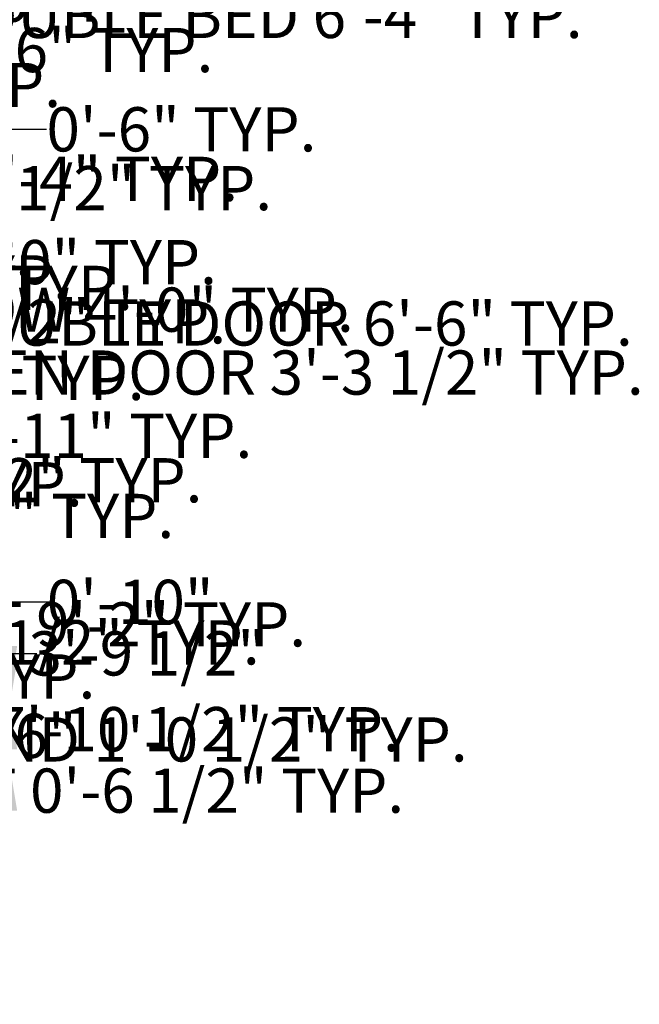
# Model space of a CAD drawing. Units: inches. Extents: x 7323 to 9737, y 2037 to 3322.
# Tile 16 of 19: x 9314 to 9737, y 2037 to 2709. Entities that reach past the tile are written whole.
import ezdxf

# ---------------------------------------------------------------- set-up
doc = ezdxf.new("R2010")
doc.units = ezdxf.units.IN
doc.header["$MEASUREMENT"] = 0
doc.layers.add('A-ANNO-DIMS', color=2, linetype='Continuous', lineweight=18)
doc.styles.get("Standard").update_dxf_attribs({"font": 'arial.ttf'})
doc.dimstyles.get("Standard").update_dxf_attribs({"dimtxt": 30.18, "dimasz": 30.18, "dimexe": 0.18, "dimexo": 0.0625, "dimgap": 0.09, "dimtad": 0, "dimtih": 1, "dimtoh": 1, "dimdec": 0, "dimzin": 0, "dimdsep": 46, "dimlunit": 3, "dimtxsty": 'Standard', "dimcen": 0.09, "dimadec": 0, "dimazin": 0, "dimtfac": 1, "dimtdec": 0, "dimtofl": 0, "dimtmove": 0, "dimatfit": 3, "dimfxl": 1, "dimtolj": 1, "dimtzin": 0, "dimarcsym": 0})

# ---------------------------------------------------------------- blocks, each defined once
blk = doc.blocks.new('*D35')
at = {"layer": 'A-ANNO-DIMS', "color": 0, "lineweight": -2, "transparency": 16777216}
for p, q in [((8977.7, 2688.2), (8947.52, 2688.2)), ((9007.88, 2687.36), (9007.88, 2688.38)), ((9013.95, 2687.36), (9013.95, 2688.38)), ((9044.13, 2688.2), (9074.31, 2688.2))]:
    blk.add_line(p, q, dxfattribs=at)
at = {"layer": 'A-ANNO-DIMS', "color": 0, "transparency": 16777216}
for points in [[(8977.7, 2693.23), (8977.7, 2683.17), (9007.88, 2688.2)], [(9044.13, 2693.23), (9044.13, 2683.17), (9013.95, 2688.2)]]:
    blk.add_solid(points, dxfattribs=at)
at = {"layer": 'Defpoints', "color": 0, "transparency": 16777216}
for p in [(9013.95, 2688.2), (9007.88, 2687.3), (9013.95, 2687.3)]:
    blk.add_point(p, dxfattribs=at)
at = {"layer": 'A-ANNO-DIMS', "color": 0, "transparency": 16777216, "insert": (9263.41, 2688.2), "char_height": 30.18, "attachment_point": 5}
blk.add_mtext('\\A1;COLUMN 0\'-6" TYP.', dxfattribs=at)
blk = doc.blocks.new('*D37')
at = {"layer": 'A-ANNO-DIMS', "color": 0, "lineweight": -2, "transparency": 16777216}
for p, q in [((9279.75, 2656.48), (9279.75, 2686.66)), ((9272.01, 2626.3), (9279.93, 2626.3)), ((9272.01, 2574.3), (9279.93, 2574.3)), ((9279.75, 2544.12), (9279.75, 2513.94))]:
    blk.add_line(p, q, dxfattribs=at)
at = {"layer": 'A-ANNO-DIMS', "color": 0, "transparency": 16777216}
for points in [[(9274.72, 2656.48), (9284.78, 2656.48), (9279.75, 2626.3)], [(9274.72, 2544.12), (9284.78, 2544.12), (9279.75, 2574.3)]]:
    blk.add_solid(points, dxfattribs=at)
at = {"layer": 'Defpoints', "color": 0, "transparency": 16777216}
for p in [(9271.95, 2626.3), (9271.95, 2574.3), (9279.75, 2574.3)]:
    blk.add_point(p, dxfattribs=at)
at = {"layer": 'A-ANNO-DIMS', "color": 0, "transparency": 16777216, "insert": (9279.75, 2600.3), "char_height": 30.18, "attachment_point": 5}
blk.add_mtext('\\A1;WINDOW 4\'-4" TYP.', dxfattribs=at)
blk = doc.blocks.new('*D38')
at = {"layer": 'A-ANNO-DIMS', "color": 0, "lineweight": -2, "transparency": 16777216}
for p, q in [((9235.77, 2634.1), (9205.59, 2634.1)), ((9265.95, 2626.36), (9265.95, 2634.28)), ((9271.95, 2626.36), (9271.95, 2634.28)), ((9302.13, 2634.1), (9332.31, 2634.1))]:
    blk.add_line(p, q, dxfattribs=at)
at = {"layer": 'A-ANNO-DIMS', "color": 0, "transparency": 16777216}
for points in [[(9235.77, 2639.13), (9235.77, 2629.07), (9265.95, 2634.1)], [(9302.13, 2639.13), (9302.13, 2629.07), (9271.95, 2634.1)]]:
    blk.add_solid(points, dxfattribs=at)
at = {"layer": 'Defpoints', "color": 0, "transparency": 16777216}
for p in [(9271.95, 2634.1), (9265.95, 2626.3), (9271.95, 2626.3)]:
    blk.add_point(p, dxfattribs=at)
at = {"layer": 'A-ANNO-DIMS', "color": 0, "transparency": 16777216, "insert": (9424.38, 2634.1), "char_height": 30.18, "attachment_point": 5}
blk.add_mtext('\\A1;0\'-6" TYP.', dxfattribs=at)
blk = doc.blocks.new('*D39')
at = {"layer": 'A-ANNO-DIMS', "color": 0, "lineweight": -2, "transparency": 16777216}
for p, q in [((8647.94, 2549.03), (8617.76, 2549.03)), ((8678.12, 2543.2), (8678.12, 2549.21)), ((8717.39, 2543.2), (8717.39, 2549.21)), ((8747.57, 2549.03), (8777.75, 2549.03))]:
    blk.add_line(p, q, dxfattribs=at)
at = {"layer": 'A-ANNO-DIMS', "color": 0, "transparency": 16777216}
for points in [[(8647.94, 2554.06), (8647.94, 2544), (8678.12, 2549.03)], [(8747.57, 2554.06), (8747.57, 2544), (8717.39, 2549.03)]]:
    blk.add_solid(points, dxfattribs=at)
at = {"layer": 'Defpoints', "color": 0, "transparency": 16777216}
for p in [(8717.39, 2549.03), (8678.12, 2543.14), (8717.39, 2543.14)]:
    blk.add_point(p, dxfattribs=at)
at = {"layer": 'A-ANNO-DIMS', "color": 0, "transparency": 16777216, "insert": (9057.19, 2549.03), "char_height": 30.18, "attachment_point": 5}
blk.add_mtext('\\A1;SINGLE DOOR 3\'-3 1/2" TYP.', dxfattribs=at)
blk = doc.blocks.new('*D43')
at = {"layer": 'A-ANNO-DIMS', "color": 0, "lineweight": -2, "transparency": 16777216}
for p, q in [((9108.94, 2438.75), (9108.94, 2468.93)), ((9104.01, 2408.57), (9109.12, 2408.57)), ((9104.01, 2375.3), (9109.12, 2375.3)), ((9108.94, 2345.12), (9108.94, 2314.94))]:
    blk.add_line(p, q, dxfattribs=at)
at = {"layer": 'A-ANNO-DIMS', "color": 0, "transparency": 16777216}
for points in [[(9103.91, 2438.75), (9113.97, 2438.75), (9108.94, 2408.57)], [(9103.91, 2345.12), (9113.97, 2345.12), (9108.94, 2375.3)]]:
    blk.add_solid(points, dxfattribs=at)
at = {"layer": 'Defpoints', "color": 0, "transparency": 16777216}
for p in [(9103.95, 2408.57), (9108.94, 2408.57), (9103.95, 2375.3)]:
    blk.add_point(p, dxfattribs=at)
at = {"layer": 'A-ANNO-DIMS', "color": 0, "transparency": 16777216, "insert": (9108.94, 2391.93), "char_height": 30.18, "attachment_point": 5}
blk.add_mtext('\\A1;BATH DOOR 2\'-9 1/2" TYP.', dxfattribs=at)
blk = doc.blocks.new('*D44')
at = {"layer": 'A-ANNO-DIMS', "color": 0, "lineweight": -2, "transparency": 16777216}
for p, q in [((9070.67, 2375.23), (9070.67, 2370.12)), ((9103.95, 2375.23), (9103.95, 2370.12)), ((9040.49, 2370.3), (9010.31, 2370.3)), ((9134.13, 2370.3), (9164.31, 2370.3))]:
    blk.add_line(p, q, dxfattribs=at)
at = {"layer": 'A-ANNO-DIMS', "color": 0, "transparency": 16777216}
for points in [[(9040.49, 2375.33), (9040.49, 2365.27), (9070.67, 2370.3)], [(9134.13, 2375.33), (9134.13, 2365.27), (9103.95, 2370.3)]]:
    blk.add_solid(points, dxfattribs=at)
at = {"layer": 'Defpoints', "color": 0, "transparency": 16777216}
for p in [(9070.67, 2375.3), (9103.95, 2375.3), (9103.95, 2370.3)]:
    blk.add_point(p, dxfattribs=at)
at = {"layer": 'A-ANNO-DIMS', "color": 0, "transparency": 16777216, "insert": (9291.8, 2370.3), "char_height": 30.18, "attachment_point": 5}
blk.add_mtext('\\A1;2\'-9 1/2" TYP.', dxfattribs=at)
blk = doc.blocks.new('*D45')
at = {"layer": 'A-ANNO-DIMS', "color": 0, "lineweight": -2, "transparency": 16777216}
for p, q in [((8725.79, 2664.36), (8695.61, 2664.36)), ((8755.97, 2662.02), (8755.97, 2664.54)), ((8772, 2662.02), (8772, 2664.54)), ((8802.18, 2664.36), (8832.36, 2664.36))]:
    blk.add_line(p, q, dxfattribs=at)
at = {"layer": 'A-ANNO-DIMS', "color": 0, "transparency": 16777216}
for points in [[(8725.79, 2669.39), (8725.79, 2659.33), (8755.97, 2664.36)], [(8802.18, 2669.39), (8802.18, 2659.33), (8772, 2664.36)]]:
    blk.add_solid(points, dxfattribs=at)
at = {"layer": 'Defpoints', "color": 0, "transparency": 16777216}
for p in [(8755.97, 2661.96), (8772, 2664.36), (8772, 2661.96)]:
    blk.add_point(p, dxfattribs=at)
at = {"layer": 'A-ANNO-DIMS', "color": 0, "transparency": 16777216, "insert": (9094.8, 2664.36), "char_height": 30.18, "attachment_point": 5}
blk.add_mtext('\\A1;BEDSIDE TABLE 1\'-4" TYP.', dxfattribs=at)
blk = doc.blocks.new('*D47')
at = {"layer": 'A-ANNO-DIMS', "color": 0, "lineweight": -2, "transparency": 16777216}
for p, q in [((8809.55, 2464.49), (8779.37, 2464.49)), ((8839.73, 2461.79), (8839.73, 2464.67)), ((8858.14, 2461.79), (8858.14, 2464.67)), ((8888.32, 2464.49), (8918.5, 2464.49))]:
    blk.add_line(p, q, dxfattribs=at)
at = {"layer": 'A-ANNO-DIMS', "color": 0, "transparency": 16777216}
for points in [[(8809.55, 2469.52), (8809.55, 2459.46), (8839.73, 2464.49)], [(8888.32, 2469.52), (8888.32, 2459.46), (8858.14, 2464.49)]]:
    blk.add_solid(points, dxfattribs=at)
at = {"layer": 'Defpoints', "color": 0, "transparency": 16777216}
for p in [(8839.73, 2461.73), (8858.14, 2464.49), (8858.14, 2461.73)]:
    blk.add_point(p, dxfattribs=at)
at = {"layer": 'A-ANNO-DIMS', "color": 0, "transparency": 16777216, "insert": (9164.9, 2464.49), "char_height": 30.18, "attachment_point": 5}
blk.add_mtext('\\A1;ARMCHAIR 1\'-6 1/2" TYP.', dxfattribs=at)
blk = doc.blocks.new('*D49')
at = {"layer": 'A-ANNO-DIMS', "color": 0, "lineweight": -2, "transparency": 16777216}
for p, q in [((8908.77, 2183.8), (8908.77, 2182.67)), ((8915.5, 2183.8), (8915.5, 2182.67)), ((8878.59, 2182.85), (8848.41, 2182.85)), ((8945.68, 2182.85), (8975.86, 2182.85))]:
    blk.add_line(p, q, dxfattribs=at)
at = {"layer": 'A-ANNO-DIMS', "color": 0, "transparency": 16777216}
for points in [[(8878.59, 2187.88), (8878.59, 2177.82), (8908.77, 2182.85)], [(8945.68, 2187.88), (8945.68, 2177.82), (8915.5, 2182.85)]]:
    blk.add_solid(points, dxfattribs=at)
at = {"layer": 'Defpoints', "color": 0, "transparency": 16777216}
for p in [(8908.77, 2183.86), (8915.5, 2183.86), (8915.5, 2182.85)]:
    blk.add_point(p, dxfattribs=at)
at = {"layer": 'A-ANNO-DIMS', "color": 0, "transparency": 16777216, "insert": (9284.58, 2182.85), "char_height": 30.18, "attachment_point": 5}
blk.add_mtext('\\A1;STAIR END POST 0\'-6 1/2" TYP.', dxfattribs=at)
blk = doc.blocks.new('*D51')
at = {"layer": 'A-ANNO-DIMS', "color": 0, "lineweight": -2, "transparency": 16777216}
for p, q in [((9130.95, 2513.23), (9130.95, 2501.42)), ((9208.95, 2513.23), (9208.95, 2501.42)), ((9161.13, 2501.6), (9178.77, 2501.6)), ((9208.95, 2501.6), (9239.13, 2501.6))]:
    blk.add_line(p, q, dxfattribs=at)
at = {"layer": 'A-ANNO-DIMS', "color": 0, "transparency": 16777216}
for points in [[(9161.13, 2506.63), (9161.13, 2496.57), (9130.95, 2501.6)], [(9178.77, 2506.63), (9178.77, 2496.57), (9208.95, 2501.6)]]:
    blk.add_solid(points, dxfattribs=at)
at = {"layer": 'Defpoints', "color": 0, "transparency": 16777216}
for p in [(9130.95, 2513.3), (9208.95, 2513.3), (9208.95, 2501.6)]:
    blk.add_point(p, dxfattribs=at)
at = {"layer": 'A-ANNO-DIMS', "color": 0, "transparency": 16777216, "insert": (9492.09, 2501.6), "char_height": 30.18, "attachment_point": 5}
blk.add_mtext('\\A1;DOUBLE DOOR 6\'-6" TYP.', dxfattribs=at)
blk = doc.blocks.new('*D52')
at = {"layer": 'A-ANNO-DIMS', "color": 0, "lineweight": -2, "transparency": 16777216}
for p, q in [((9220.65, 2583.03), (9220.65, 2613.21)), ((9209.01, 2552.85), (9220.83, 2552.85)), ((9209.01, 2513.3), (9220.83, 2513.3)), ((9220.65, 2483.12), (9220.65, 2452.94))]:
    blk.add_line(p, q, dxfattribs=at)
at = {"layer": 'A-ANNO-DIMS', "color": 0, "transparency": 16777216}
for points in [[(9215.62, 2583.03), (9225.68, 2583.03), (9220.65, 2552.85)], [(9215.62, 2483.12), (9225.68, 2483.12), (9220.65, 2513.3)]]:
    blk.add_solid(points, dxfattribs=at)
at = {"layer": 'Defpoints', "color": 0, "transparency": 16777216}
for p in [(9208.95, 2552.85), (9220.65, 2552.85), (9208.95, 2513.3)]:
    blk.add_point(p, dxfattribs=at)
at = {"layer": 'A-ANNO-DIMS', "color": 0, "transparency": 16777216, "insert": (9220.65, 2533.07), "char_height": 30.18, "attachment_point": 5}
blk.add_mtext('\\A1;3\'-3 1/2" TYP.', dxfattribs=at)
blk = doc.blocks.new('*D53')
at = {"layer": 'A-ANNO-DIMS', "color": 0, "lineweight": -2, "transparency": 16777216}
for p, q in [((8826.85, 2511.06), (8796.67, 2511.06)), ((8857.03, 2503.93), (8857.03, 2511.24)), ((8905.03, 2503.93), (8905.03, 2511.24)), ((8935.21, 2511.06), (8965.39, 2511.06))]:
    blk.add_line(p, q, dxfattribs=at)
at = {"layer": 'A-ANNO-DIMS', "color": 0, "transparency": 16777216}
for points in [[(8826.85, 2516.09), (8826.85, 2506.03), (8857.03, 2511.06)], [(8935.21, 2516.09), (8935.21, 2506.03), (8905.03, 2511.06)]]:
    blk.add_solid(points, dxfattribs=at)
at = {"layer": 'Defpoints', "color": 0, "transparency": 16777216}
for p in [(8905.03, 2511.06), (8857.03, 2503.86), (8905.03, 2503.86)]:
    blk.add_point(p, dxfattribs=at)
at = {"layer": 'A-ANNO-DIMS', "color": 0, "transparency": 16777216, "insert": (9261.3, 2511.06), "char_height": 30.18, "attachment_point": 5}
blk.add_mtext('\\A1;INTERIOR WINDOW 4\'-0" TYP.', dxfattribs=at)
blk = doc.blocks.new('*D55')
at = {"layer": 'A-ANNO-DIMS', "color": 0, "lineweight": -2, "transparency": 16777216}
for p, q in [((9265.38, 2351.3), (9282, 2351.3)), ((9281.82, 2321.12), (9281.82, 2311.99)), ((9281.82, 2271.48), (9281.82, 2280.6)), ((9265.38, 2241.3), (9282, 2241.3))]:
    blk.add_line(p, q, dxfattribs=at)
at = {"layer": 'A-ANNO-DIMS', "color": 0, "transparency": 16777216}
for points in [[(9276.79, 2321.12), (9286.85, 2321.12), (9281.82, 2351.3)], [(9276.79, 2271.48), (9286.85, 2271.48), (9281.82, 2241.3)]]:
    blk.add_solid(points, dxfattribs=at)
at = {"layer": 'Defpoints', "color": 0, "transparency": 16777216}
for p in [(9265.32, 2351.3), (9281.82, 2351.3), (9265.32, 2241.3)]:
    blk.add_point(p, dxfattribs=at)
at = {"layer": 'A-ANNO-DIMS', "color": 0, "transparency": 16777216, "insert": (9281.82, 2296.3), "char_height": 30.18, "attachment_point": 5}
blk.add_mtext('\\A1;STAIR FLIGHT 9\'-2" TYP.', dxfattribs=at)
blk = doc.blocks.new('*D56')
at = {"layer": 'A-ANNO-DIMS', "color": 0, "lineweight": -2, "transparency": 16777216}
for p, q in [((9170.68, 2241.23), (9170.68, 2224.62)), ((9265.32, 2241.23), (9265.32, 2224.62)), ((9200.86, 2224.8), (9235.14, 2224.8)), ((9265.32, 2224.8), (9295.5, 2224.8))]:
    blk.add_line(p, q, dxfattribs=at)
at = {"layer": 'A-ANNO-DIMS', "color": 0, "transparency": 16777216}
for points in [[(9200.86, 2229.83), (9200.86, 2219.77), (9170.68, 2224.8)], [(9235.14, 2229.83), (9235.14, 2219.77), (9265.32, 2224.8)]]:
    blk.add_solid(points, dxfattribs=at)
at = {"layer": 'Defpoints', "color": 0, "transparency": 16777216}
for p in [(9170.68, 2241.3), (9265.32, 2241.3), (9265.32, 2224.8)]:
    blk.add_point(p, dxfattribs=at)
at = {"layer": 'A-ANNO-DIMS', "color": 0, "transparency": 16777216, "insert": (9434.33, 2224.8), "char_height": 30.18, "attachment_point": 5}
blk.add_mtext('\\A1;7\'-10 1/2" TYP.', dxfattribs=at)
blk = doc.blocks.new('*D59')
at = {"layer": 'A-ANNO-DIMS', "color": 0, "lineweight": -2, "transparency": 16777216}
for p, q in [((9064.67, 2473.96), (9064.67, 2467.95)), ((9103.95, 2473.96), (9103.95, 2467.95)), ((9034.49, 2468.13), (9004.31, 2468.13)), ((9134.13, 2468.13), (9164.31, 2468.13))]:
    blk.add_line(p, q, dxfattribs=at)
at = {"layer": 'A-ANNO-DIMS', "color": 0, "transparency": 16777216}
for points in [[(9034.49, 2473.16), (9034.49, 2463.1), (9064.67, 2468.13)], [(9134.13, 2473.16), (9134.13, 2463.1), (9103.95, 2468.13)]]:
    blk.add_solid(points, dxfattribs=at)
at = {"layer": 'Defpoints', "color": 0, "transparency": 16777216}
for p in [(9064.67, 2474.02), (9103.95, 2474.02), (9103.95, 2468.13)]:
    blk.add_point(p, dxfattribs=at)
at = {"layer": 'A-ANNO-DIMS', "color": 0, "transparency": 16777216, "insert": (9458.35, 2468.13), "char_height": 30.18, "attachment_point": 5}
blk.add_mtext('\\A1;KITCHEN DOOR 3\'-3 1/2" TYP.', dxfattribs=at)
blk = doc.blocks.new('*D61')
at = {"layer": 'A-ANNO-DIMS', "color": 0, "lineweight": -2, "transparency": 16777216}
for p, q in [((9212.57, 2681.3), (9212.57, 2711.48)), ((9212.57, 2711.48), (9242.75, 2711.48)), ((9201.24, 2681.3), (9212.75, 2681.3)), ((9212.57, 2635.56), (9212.57, 2651.12)), ((9201.24, 2605.38), (9212.75, 2605.38))]:
    blk.add_line(p, q, dxfattribs=at)
at = {"layer": 'A-ANNO-DIMS', "color": 0, "transparency": 16777216}
for points in [[(9207.54, 2651.12), (9217.6, 2651.12), (9212.57, 2681.3)], [(9207.54, 2635.56), (9217.6, 2635.56), (9212.57, 2605.38)]]:
    blk.add_solid(points, dxfattribs=at)
at = {"layer": 'Defpoints', "color": 0, "transparency": 16777216}
for p in [(9201.18, 2681.3), (9212.57, 2681.3), (9201.18, 2605.38)]:
    blk.add_point(p, dxfattribs=at)
at = {"layer": 'A-ANNO-DIMS', "color": 0, "transparency": 16777216, "insert": (9475.82, 2711.48), "char_height": 30.18, "attachment_point": 5}
blk.add_mtext('\\A1;DOUBLE BED 6\'-4" TYP.', dxfattribs=at)
blk = doc.blocks.new('*D62')
at = {"layer": 'A-ANNO-DIMS', "color": 0, "lineweight": -2, "transparency": 16777216}
for p, q in [((9134.53, 2605.32), (9134.53, 2593.82)), ((9201.18, 2605.32), (9201.18, 2593.82)), ((9164.71, 2594), (9171, 2594)), ((9201.18, 2594), (9231.36, 2594))]:
    blk.add_line(p, q, dxfattribs=at)
at = {"layer": 'A-ANNO-DIMS', "color": 0, "transparency": 16777216}
for points in [[(9164.71, 2599.03), (9164.71, 2588.97), (9134.53, 2594)], [(9171, 2599.03), (9171, 2588.97), (9201.18, 2594)]]:
    blk.add_solid(points, dxfattribs=at)
at = {"layer": 'Defpoints', "color": 0, "transparency": 16777216}
for p in [(9134.53, 2605.38), (9201.18, 2605.38), (9201.18, 2594)]:
    blk.add_point(p, dxfattribs=at)
at = {"layer": 'A-ANNO-DIMS', "color": 0, "transparency": 16777216, "insert": (9358.59, 2594), "char_height": 30.18, "attachment_point": 5}
blk.add_mtext('\\A1;5\'-6 1/2" TYP.', dxfattribs=at)
blk = doc.blocks.new('*D65')
at = {"layer": 'A-ANNO-DIMS', "color": 0, "lineweight": -2, "transparency": 16777216}
for p, q in [((9024.02, 2513.3), (9024.02, 2543.48)), ((9024.02, 2543.48), (9054.2, 2543.48)), ((9036.56, 2513.3), (9023.84, 2513.3)), ((9024.02, 2459.48), (9024.02, 2483.12)), ((9036.56, 2429.3), (9023.84, 2429.3))]:
    blk.add_line(p, q, dxfattribs=at)
at = {"layer": 'A-ANNO-DIMS', "color": 0, "transparency": 16777216}
for points in [[(9018.99, 2483.12), (9029.05, 2483.12), (9024.02, 2513.3)], [(9018.99, 2459.48), (9029.05, 2459.48), (9024.02, 2429.3)]]:
    blk.add_solid(points, dxfattribs=at)
at = {"layer": 'Defpoints', "color": 0, "transparency": 16777216}
for p in [(9024.02, 2513.3), (9036.62, 2513.3), (9036.62, 2429.3)]:
    blk.add_point(p, dxfattribs=at)
at = {"layer": 'A-ANNO-DIMS', "color": 0, "transparency": 16777216, "insert": (9256.18, 2543.48), "char_height": 30.18, "attachment_point": 5}
blk.add_mtext('\\A1;COUNTER 7\'-0" TYP.', dxfattribs=at)
blk = doc.blocks.new('*D66')
at = {"layer": 'A-ANNO-DIMS', "color": 0, "lineweight": -2, "transparency": 16777216}
for p, q in [((9006.44, 2525.9), (8976.26, 2525.9)), ((9036.62, 2513.36), (9036.62, 2526.08)), ((9075.95, 2513.36), (9075.95, 2526.08)), ((9106.13, 2525.9), (9136.31, 2525.9))]:
    blk.add_line(p, q, dxfattribs=at)
at = {"layer": 'A-ANNO-DIMS', "color": 0, "transparency": 16777216}
for points in [[(9006.44, 2530.93), (9006.44, 2520.87), (9036.62, 2525.9)], [(9106.13, 2530.93), (9106.13, 2520.87), (9075.95, 2525.9)]]:
    blk.add_solid(points, dxfattribs=at)
at = {"layer": 'Defpoints', "color": 0, "transparency": 16777216}
for p in [(9075.95, 2525.9), (9036.62, 2513.3), (9075.95, 2513.3)]:
    blk.add_point(p, dxfattribs=at)
at = {"layer": 'A-ANNO-DIMS', "color": 0, "transparency": 16777216, "insert": (9263.53, 2525.9), "char_height": 30.18, "attachment_point": 5}
blk.add_mtext('\\A1;3\'-3 1/2" TYP.', dxfattribs=at)
blk = doc.blocks.new('*D67')
at = {"layer": 'A-ANNO-DIMS', "color": 0, "lineweight": -2, "transparency": 16777216}
for p, q in [((9145.07, 2308.82), (9145.07, 2339)), ((9150.37, 2278.64), (9144.89, 2278.64)), ((9150.37, 2242.89), (9144.89, 2242.89)), ((9145.07, 2212.71), (9145.07, 2182.53))]:
    blk.add_line(p, q, dxfattribs=at)
at = {"layer": 'A-ANNO-DIMS', "color": 0, "transparency": 16777216}
for points in [[(9140.04, 2308.82), (9150.1, 2308.82), (9145.07, 2278.64)], [(9140.04, 2212.71), (9150.1, 2212.71), (9145.07, 2242.89)]]:
    blk.add_solid(points, dxfattribs=at)
at = {"layer": 'Defpoints', "color": 0, "transparency": 16777216}
for p in [(9145.07, 2278.64), (9150.44, 2278.64), (9150.44, 2242.89)]:
    blk.add_point(p, dxfattribs=at)
at = {"layer": 'A-ANNO-DIMS', "color": 0, "transparency": 16777216, "insert": (9145.07, 2260.76), "char_height": 30.18, "attachment_point": 5}
blk.add_mtext('\\A1;TV UNIT 2\'-11 1/2" TYP.', dxfattribs=at)
blk = doc.blocks.new('*D68')
at = {"layer": 'A-ANNO-DIMS', "color": 0, "lineweight": -2, "transparency": 16777216}
for p, q in [((9120.26, 2284), (9090.08, 2284)), ((9150.44, 2278.7), (9150.44, 2284.18)), ((9163.95, 2278.7), (9163.95, 2284.18)), ((9194.13, 2284), (9224.31, 2284))]:
    blk.add_line(p, q, dxfattribs=at)
at = {"layer": 'A-ANNO-DIMS', "color": 0, "transparency": 16777216}
for points in [[(9120.26, 2289.03), (9120.26, 2278.97), (9150.44, 2284)], [(9194.13, 2289.03), (9194.13, 2278.97), (9163.95, 2284)]]:
    blk.add_solid(points, dxfattribs=at)
at = {"layer": 'Defpoints', "color": 0, "transparency": 16777216}
for p in [(9150.44, 2278.64), (9163.95, 2284), (9163.95, 2278.64)]:
    blk.add_point(p, dxfattribs=at)
at = {"layer": 'A-ANNO-DIMS', "color": 0, "transparency": 16777216, "insert": (9350.12, 2284), "char_height": 30.18, "attachment_point": 5}
blk.add_mtext('\\A1;1\'-1 1/2" TYP.', dxfattribs=at)
blk = doc.blocks.new('*D69')
at = {"layer": 'A-ANNO-DIMS', "color": 0, "lineweight": -2, "transparency": 16777216}
for p, q in [((8836.58, 2472.89), (8836.58, 2503.07)), ((8836.58, 2503.07), (8866.76, 2503.07)), ((8839.88, 2442.71), (8836.4, 2442.71)), ((8839.88, 2420.33), (8836.4, 2420.33)), ((8836.58, 2390.15), (8836.58, 2359.97))]:
    blk.add_line(p, q, dxfattribs=at)
at = {"layer": 'A-ANNO-DIMS', "color": 0, "transparency": 16777216}
for points in [[(8831.55, 2472.89), (8841.61, 2472.89), (8836.58, 2442.71)], [(8831.55, 2390.15), (8841.61, 2390.15), (8836.58, 2420.33)]]:
    blk.add_solid(points, dxfattribs=at)
at = {"layer": 'Defpoints', "color": 0, "transparency": 16777216}
for p in [(8836.58, 2442.71), (8839.94, 2442.71), (8839.94, 2420.33)]:
    blk.add_point(p, dxfattribs=at)
at = {"layer": 'A-ANNO-DIMS', "color": 0, "transparency": 16777216, "insert": (9169.54, 2503.07), "char_height": 30.18, "attachment_point": 5}
blk.add_mtext('\\A1;COFFEE TABLE 1\'-10 1/2" TYP.', dxfattribs=at)
blk = doc.blocks.new('*D73')
at = {"layer": 'A-ANNO-DIMS', "color": 0, "lineweight": -2, "transparency": 16777216}
for p, q in [((9031.41, 2424.97), (9001.23, 2424.97)), ((9061.59, 2423.36), (9061.59, 2425.15)), ((9072.75, 2423.36), (9072.75, 2425.15)), ((9102.93, 2424.97), (9133.11, 2424.97))]:
    blk.add_line(p, q, dxfattribs=at)
at = {"layer": 'A-ANNO-DIMS', "color": 0, "transparency": 16777216}
for points in [[(9031.41, 2430), (9031.41, 2419.94), (9061.59, 2424.97)], [(9102.93, 2430), (9102.93, 2419.94), (9072.75, 2424.97)]]:
    blk.add_solid(points, dxfattribs=at)
at = {"layer": 'Defpoints', "color": 0, "transparency": 16777216}
for p in [(9061.59, 2423.3), (9072.75, 2424.97), (9072.75, 2423.3)]:
    blk.add_point(p, dxfattribs=at)
at = {"layer": 'A-ANNO-DIMS', "color": 0, "transparency": 16777216, "insert": (9305.36, 2424.97), "char_height": 30.18, "attachment_point": 5}
blk.add_mtext('\\A1;BASIN 0\'-11" TYP.', dxfattribs=at)
blk = doc.blocks.new('*D77')
at = {"layer": 'A-ANNO-DIMS', "color": 0, "lineweight": -2, "transparency": 16777216}
for p, q in [((8986.18, 2217.79), (8956, 2217.79)), ((9016.36, 2219.63), (9016.36, 2217.61)), ((9029.07, 2219.63), (9029.07, 2217.61)), ((9059.25, 2217.79), (9089.43, 2217.79))]:
    blk.add_line(p, q, dxfattribs=at)
at = {"layer": 'A-ANNO-DIMS', "color": 0, "transparency": 16777216}
for points in [[(8986.18, 2222.82), (8986.18, 2212.76), (9016.36, 2217.79)], [(9059.25, 2222.82), (9059.25, 2212.76), (9029.07, 2217.79)]]:
    blk.add_solid(points, dxfattribs=at)
at = {"layer": 'Defpoints', "color": 0, "transparency": 16777216}
for p in [(9016.36, 2219.69), (9029.07, 2219.69), (9029.07, 2217.79)]:
    blk.add_point(p, dxfattribs=at)
at = {"layer": 'A-ANNO-DIMS', "color": 0, "transparency": 16777216, "insert": (9358.82, 2217.79), "char_height": 30.18, "attachment_point": 5}
blk.add_mtext('\\A1;NIGHTSTAND 1\'-0 1/2" TYP.', dxfattribs=at)
blk = doc.blocks.new('*D79')
at = {"layer": 'A-ANNO-DIMS', "color": 0, "lineweight": -2, "transparency": 16777216}
for p, q in [((8840.92, 2394.64), (8810.74, 2394.64)), ((8871.1, 2395.97), (8871.1, 2394.46)), ((8880.36, 2395.97), (8880.36, 2394.46)), ((8910.54, 2394.64), (8940.72, 2394.64))]:
    blk.add_line(p, q, dxfattribs=at)
at = {"layer": 'A-ANNO-DIMS', "color": 0, "transparency": 16777216}
for points in [[(8840.92, 2399.67), (8840.92, 2389.61), (8871.1, 2394.64)], [(8910.54, 2399.67), (8910.54, 2389.61), (8880.36, 2394.64)]]:
    blk.add_solid(points, dxfattribs=at)
at = {"layer": 'Defpoints', "color": 0, "transparency": 16777216}
for p in [(8871.1, 2396.03), (8880.36, 2396.03), (8880.36, 2394.64)]:
    blk.add_point(p, dxfattribs=at)
at = {"layer": 'A-ANNO-DIMS', "color": 0, "transparency": 16777216, "insert": (9195.57, 2394.64), "char_height": 30.18, "attachment_point": 5}
blk.add_mtext('\\A1;SIDE TABLE 0\'-9 1/2" TYP.', dxfattribs=at)
blk = doc.blocks.new('*D115')
at = {"layer": 'A-ANNO-DIMS', "color": 0, "lineweight": -2, "transparency": 16777216}
for p, q in [((9307.269962, 2271.475205), (9307.269962, 2301.655205)), ((9265.38043, 2241.295205), (9307.449962, 2241.295205)), ((9265.38043, 2199.295205), (9307.449962, 2199.295205)), ((9307.269962, 2169.115205), (9307.269962, 2138.935205))]:
    blk.add_line(p, q, dxfattribs=at)
at = {"layer": 'A-ANNO-DIMS', "color": 0, "transparency": 16777216}
for points in [[(9302.239962, 2271.475205), (9312.299962, 2271.475205), (9307.269962, 2241.295205)], [(9302.239962, 2169.115205), (9312.299962, 2169.115205), (9307.269962, 2199.295205)]]:
    blk.add_solid(points, dxfattribs=at)
at = {"layer": 'Defpoints', "color": 0, "transparency": 16777216}
for p in [(9265.31793, 2241.295205), (9307.269962, 2241.295205), (9265.31793, 2199.295205)]:
    blk.add_point(p, dxfattribs=at)
at = {"layer": 'A-ANNO-DIMS', "color": 0, "transparency": 16777216, "insert": (9307.269962, 2220.295205), "char_height": 30.18, "attachment_point": 5}
blk.add_mtext('\\A1;3\'-6"', dxfattribs=at)
blk = doc.blocks.new('*D116')
at = {"layer": 'A-ANNO-DIMS', "color": 0, "lineweight": -2, "transparency": 16777216}
for p, q in [((9307.27, 2281.48), (9307.27, 2311.66)), ((9307.27, 2311.66), (9337.45, 2311.66)), ((9265.38, 2251.3), (9307.45, 2251.3)), ((9265.38, 2241.3), (9307.45, 2241.3)), ((9307.27, 2211.12), (9307.27, 2180.94))]:
    blk.add_line(p, q, dxfattribs=at)
at = {"layer": 'A-ANNO-DIMS', "color": 0, "transparency": 16777216}
for points in [[(9302.24, 2281.48), (9312.3, 2281.48), (9307.27, 2251.3)], [(9302.24, 2211.12), (9312.3, 2211.12), (9307.27, 2241.3)]]:
    blk.add_solid(points, dxfattribs=at)
at = {"layer": 'Defpoints', "color": 0, "transparency": 16777216}
for p in [(9265.32, 2251.3), (9307.27, 2251.3), (9265.32, 2241.3)]:
    blk.add_point(p, dxfattribs=at)
at = {"layer": 'A-ANNO-DIMS', "color": 0, "transparency": 16777216, "insert": (9389.38, 2311.66), "char_height": 30.18, "attachment_point": 5}
blk.add_mtext('\\A1;0\'-10"', dxfattribs=at)
blk = doc.blocks.new('*D122')
at = {"layer": 'A-ANNO-DIMS', "color": 0, "lineweight": -2, "transparency": 16777216}
for p, q in [((9189.82, 2276.5), (9159.64, 2276.5)), ((9220, 2241.36), (9220, 2276.68)), ((9265.32, 2241.36), (9265.32, 2276.68)), ((9295.5, 2276.5), (9325.68, 2276.5))]:
    blk.add_line(p, q, dxfattribs=at)
at = {"layer": 'A-ANNO-DIMS', "color": 0, "transparency": 16777216}
for points in [[(9189.82, 2281.53), (9189.82, 2271.47), (9220, 2276.5)], [(9295.5, 2281.53), (9295.5, 2271.47), (9265.32, 2276.5)]]:
    blk.add_solid(points, dxfattribs=at)
at = {"layer": 'Defpoints', "color": 0, "transparency": 16777216}
for p in [(9265.32, 2276.5), (9220, 2241.3), (9265.32, 2241.3)]:
    blk.add_point(p, dxfattribs=at)
at = {"layer": 'A-ANNO-DIMS', "color": 0, "transparency": 16777216, "insert": (9401.03, 2276.5), "char_height": 30.18, "attachment_point": 5}
blk.add_mtext('\\A1;3\'-9 1/2"', dxfattribs=at)
blk = doc.blocks.new('*D123')
at = {"layer": 'A-ANNO-DIMS', "color": 0, "lineweight": -2, "transparency": 16777216}
for p, q in [((9195.95, 2687.36), (9195.95, 2722.73)), ((9226.13, 2722.55), (9241.77, 2722.55)), ((9271.95, 2687.36), (9271.95, 2722.73)), ((9271.95, 2722.55), (9302.13, 2722.55))]:
    blk.add_line(p, q, dxfattribs=at)
at = {"layer": 'A-ANNO-DIMS', "color": 0, "transparency": 16777216}
for points in [[(9226.13, 2727.58), (9226.13, 2717.52), (9195.95, 2722.55)], [(9241.77, 2727.58), (9241.77, 2717.52), (9271.95, 2722.55)]]:
    blk.add_solid(points, dxfattribs=at)
at = {"layer": 'Defpoints', "color": 0, "transparency": 16777216}
for p in [(9271.95, 2722.55), (9195.95, 2687.3), (9271.95, 2687.3)]:
    blk.add_point(p, dxfattribs=at)
at = {"layer": 'A-ANNO-DIMS', "color": 0, "transparency": 16777216, "insert": (9342.41, 2722.55), "char_height": 30.18, "attachment_point": 5}
blk.add_mtext('\\A1;6\'-4"', dxfattribs=at)

msp = doc.modelspace()

# ---------------------------------------------------------------- dimensions: what is measured, and where the dimension line sits
at = {"layer": 'A-ANNO-DIMS'}
for base, p1, p2, angle, text, picture, middle in [((9212.57, 2681.3), (9201.18, 2605.38), (9201.18, 2681.3), 90, 'DOUBLE BED <> TYP.', '*D61', (9475.82, 2711.48)), ((9279.75, 2574.3), (9271.95, 2626.3), (9271.95, 2574.3), 270, 'WINDOW <> TYP.', '*D37', (9279.75, 2600.3)), ((9271.95, 2634.1), (9265.95, 2626.3), (9271.95, 2626.3), 0, '<> TYP.', '*D38', (9424.38, 2634.1)), ((8836.58, 2442.71), (8839.94, 2420.33), (8839.94, 2442.71), 90, 'COFFEE TABLE <> TYP.', '*D69', (9169.54, 2503.07)), ((9024.02, 2513.3), (9036.62, 2429.3), (9036.62, 2513.3), 90, 'COUNTER <> TYP.', '*D65', (9256.18, 2543.48)), ((9220.6454, 2552.8475), (9208.9454, 2513.2952), (9208.9454, 2552.8475), 90, '<> TYP.', '*D52', (9220.6454, 2533.0713)), ((9108.94, 2408.57), (9103.95, 2375.3), (9103.95, 2408.57), 90, 'BATH DOOR <> TYP.', '*D43', (9108.94, 2391.93)), ((9281.82, 2351.3), (9265.32, 2241.3), (9265.32, 2351.3), 90, 'STAIR FLIGHT <> TYP.', '*D55', (9281.82, 2296.3)), ((9145.0746, 2278.635), (9150.4365, 2242.8889), (9150.4365, 2278.635), 90, 'TV UNIT <> TYP.', '*D67', (9145.0746, 2260.762))]:
    dim = msp.add_linear_dim(base=base, p1=p1, p2=p2, angle=angle, text=text, dimstyle='Standard', override={"dimdec": 1, "dimlfac": 1, "dimrnd": 0, "dimzin": 1, "dimdsep": 46, "dimlunit": 4, "dimfrac": 2}, dxfattribs=at)
    dim.commit()
    dim.dimension.update_dxf_attribs({"geometry": picture, "text_midpoint": middle})
for base, p1, p2, text, picture, middle in [((8772, 2664.36), (8755.97, 2661.96), (8772, 2661.96), 'BEDSIDE TABLE <> TYP.', '*D45', (9094.8, 2664.36)), ((9013.95, 2688.2), (9007.88, 2687.3), (9013.95, 2687.3), 'COLUMN <> TYP.', '*D35', (9263.41, 2688.2)), ((8717.39, 2549.03), (8678.12, 2543.14), (8717.39, 2543.14), 'SINGLE DOOR <> TYP.', '*D39', (9057.19, 2549.03)), ((9201.1793, 2593.9956), (9134.5282, 2605.3825), (9201.1793, 2605.3825), '<> TYP.', '*D62', (9358.5924, 2593.9956)), ((8905.03, 2511.06), (8857.03, 2503.86), (8905.03, 2503.86), 'INTERIOR WINDOW <> TYP.', '*D53', (9261.3, 2511.06)), ((9075.95, 2525.9), (9036.62, 2513.3), (9075.95, 2513.3), '<> TYP.', '*D66', (9263.53, 2525.9)), ((9208.95, 2501.6), (9130.95, 2513.3), (9208.95, 2513.3), 'DOUBLE DOOR <> TYP.', '*D51', (9492.09, 2501.6)), ((9103.95, 2468.13), (9064.67, 2474.02), (9103.95, 2474.02), 'KITCHEN DOOR <> TYP.', '*D59', (9458.35, 2468.13)), ((8858.14, 2464.49), (8839.73, 2461.73), (8858.14, 2461.73), 'ARMCHAIR <> TYP.', '*D47', (9164.9, 2464.49)), ((8880.36, 2394.64), (8871.1, 2396.03), (8880.36, 2396.03), 'SIDE TABLE <> TYP.', '*D79', (9195.57, 2394.64)), ((9072.75, 2424.97), (9061.59, 2423.3), (9072.75, 2423.3), 'BASIN <> TYP.', '*D73', (9305.36, 2424.97)), ((9103.95, 2370.3), (9070.67, 2375.3), (9103.95, 2375.3), '<> TYP.', '*D44', (9291.8, 2370.3)), ((9163.95, 2284), (9150.44, 2278.64), (9163.95, 2278.64), '<> TYP.', '*D68', (9350.12, 2284)), ((8915.5, 2182.85), (8908.77, 2183.86), (8915.5, 2183.86), 'STAIR END POST <> TYP.', '*D49', (9284.58, 2182.85)), ((9029.07, 2217.79), (9016.36, 2219.69), (9029.07, 2219.69), 'NIGHTSTAND <> TYP.', '*D77', (9358.82, 2217.79)), ((9265.32, 2224.8), (9170.68, 2241.3), (9265.32, 2241.3), '<> TYP.', '*D56', (9434.33, 2224.8))]:
    dim = msp.add_linear_dim(base=base, p1=p1, p2=p2, text=text, dimstyle='Standard', override={"dimdec": 1, "dimlfac": 1, "dimrnd": 0, "dimzin": 1, "dimdsep": 46, "dimlunit": 4, "dimfrac": 2}, dxfattribs=at)
    dim.commit()
    dim.dimension.update_dxf_attribs({"geometry": picture, "text_midpoint": middle})
for base, p1, p2, picture, middle in [((9271.95, 2722.55), (9195.95, 2687.3), (9271.95, 2687.3), '*D123', (9342.41, 2722.55)), ((9265.32, 2276.5), (9220, 2241.3), (9265.32, 2241.3), '*D122', (9401.03, 2276.5))]:
    dim = msp.add_linear_dim(base=base, p1=p1, p2=p2, dimstyle='Standard', override={"dimdec": 1, "dimlfac": 1, "dimrnd": 0, "dimzin": 1, "dimdsep": 46, "dimlunit": 4, "dimfrac": 2}, dxfattribs=at)
    dim.commit()
    dim.dimension.update_dxf_attribs({"geometry": picture, "text_midpoint": middle})
for base, p1, p2, picture, middle in [((9307.27, 2251.3), (9265.32, 2241.3), (9265.32, 2251.3), '*D116', (9389.38, 2311.66)), ((9307.27, 2241.3), (9265.32, 2199.3), (9265.32, 2241.3), '*D115', (9307.27, 2220.3))]:
    dim = msp.add_linear_dim(base=base, p1=p1, p2=p2, angle=90, dimstyle='Standard', override={"dimdec": 1, "dimlfac": 1, "dimrnd": 0, "dimzin": 1, "dimdsep": 46, "dimlunit": 4, "dimfrac": 2}, dxfattribs=at)
    dim.commit()
    dim.dimension.update_dxf_attribs({"geometry": picture, "text_midpoint": middle})

doc.saveas('drawing.dxf')
